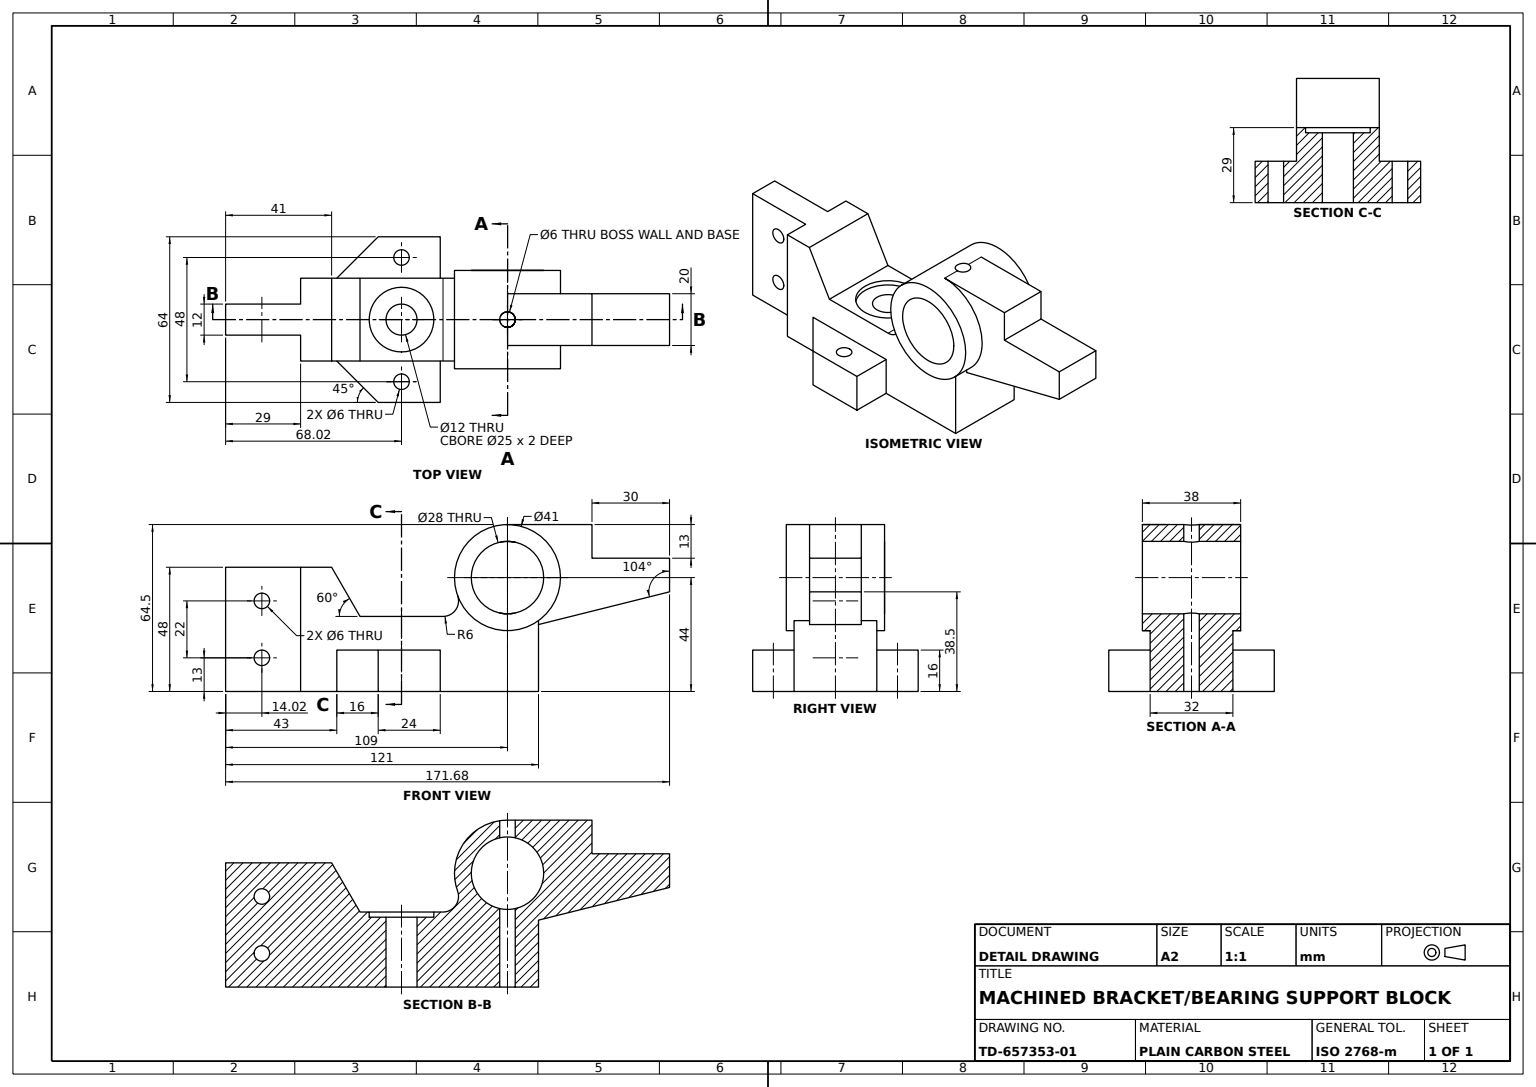
SolidWorks part; units mm, degrees
material "Plain Carbon Steel"
ref_plane "Front Plane" through (0, 0, 0) normal (0, 0, 1) x (1, 0, 0)
ref_plane "Top Plane" through (0, 0, 0) normal (0, 1, 0) x (1, 0, 0)
ref_plane "Right Plane" through (0, 0, 0) normal (1, 0, 0) x (0, 0, -1)
sketch "Base Block Sketch" plane through (0, 0, 0) normal (0, 0, 1) x (1, 0, 0)
  line L1 (-60.5, 24) -> (60.5, 24)
  line L2 (-60.5, 24) -> (-60.5, -24)
  line L3 (-60.5, -24) -> (60.5, -24)
  line L4 (60.5, 24) -> (60.5, -24)
  point P4 (0, -24)
  point P6 (-60.5, 0)
  dimension "D1" = 121
  dimension "D2" = 48
extrude "Base Block 121x48" add sketch "Base Block Sketch" along normal mid plane 32
sketch "Base Step Sketch" plane through (60.5, 0, 0) normal (1, 0, 0) x (0, 0, -1)
  line L0 (-16, -24) -> (16, -24) construction
  line L1 (-16, 24) -> (-6, 24)
  line L2 (-16, 24) -> (-16, -24)
  line L3 (-16, -24) -> (-6, -24)
  line L4 (-6, 24) -> (-6, -24)
  line L5 (0, 0) -> (0, 24) construction
  line L6 (16, 24) -> (6, 24)
  line L7 (16, 24) -> (16, -24)
  line L8 (16, -24) -> (6, -24)
  line L9 (6, 24) -> (6, -24)
  line L10 (-16, 24) -> (16, 24) construction
  dimension "D1" = 12
extrude "Base Step Cut" cut sketch "Base Step Sketch" against normal blind 29
sketch "Angled Relief Sketch" plane through (0, 0, 16) normal (0, 0, 1) x (1, 0, 0)
  line L0 (-60.5, 24) -> (-60.5, -24) construction
  line L1 (31.5, 24) -> (-60.5, 24) construction
  line L2 (19.5, 24) -> (8.5303, 5)
  line L3 (8.5303, 5) -> (-40, 5)
  line L4 (-40, 5) -> (-40, 24)
  line L5 (-60.5, -24) -> (31.5, -24) construction
  line L6 (31.5, 24) -> (31.5, -24) construction
  line L7 (-40, 24) -> (19.5, 24)
  dimension "D1" = 29
  dimension "D2" = 30
  dimension "D3" = 12
  dimension "D4" = 20.5
extrude "Angled Relief Cut 30deg" cut sketch "Angled Relief Sketch" against normal through all both and the other way through all
sketch "Pivot Boss Sketch" plane through (0, 0, 0) normal (0, 0, 1) x (1, 0, 0)
  line L0 (-60.5, -24) -> (31.5, -24) construction
  line L2 (-60.5, 24) -> (-60.5, -24) construction
  circle A0 centre (-48.5, 20) radius 20.5
  dimension "D3" = 41
  dimension "D1" = 44
  dimension "D2" = 12
extrude "Pivot Boss Ø44" add sketch "Pivot Boss Sketch" along normal mid plane 38
fillet "Pivot Boss Fillet R6" radius 6 1 edges at (-34.5268, 5, 0)
sketch "Clamp Tab Sketch" plane through (0, 0, 0) normal (0, 0, 1) x (1, 0, 0)
  line L0 (-48.5, 40.5) -> (-81.1788, 40.5)
  line L1 (-81.1788, 40.5) -> (-81.1788, 27.5)
  line L2 (-81.1788, 27.5) -> (-111.1788, 27.5)
  line L3 (-111.1788, 27.5) -> (-111.1788, 14.5)
  line L4 (-111.1788, 14.5) -> (-53.4594, 0.1089)
  circle A0 centre (-48.5, 20) radius 20.5 construction
  arc A1 (-48.5, 40.5) -> (-53.4594, 0.1089) centre (-48.5, 20) ccw
  dimension "D1" = 13
  dimension "D2" = 13
  dimension "D3" = 104
  dimension "D4" = 30
extrude "Clamp Tab" add sketch "Clamp Tab Sketch" along normal mid plane 20
sketch "Tab Pin Hole Sketch" plane through (0, 0, 0) normal (0, 1, 0) x (1, 0, 0)
  line L0 (-48.5, -10) -> (-48.5, 10) construction
  circle A0 centre (-48.5, 0) radius 3
  dimension "D1" = 6
extrude "Tab Pin Hole Ø6" cut sketch "Tab Pin Hole Sketch" against normal through all both and the other way through all
sketch "Pivot Bore Sketch" plane through (0, 0, 19) normal (0, 0, 1) x (1, 0, 0)
  circle A0 centre (-48.5, 20) radius 14
  dimension "D1" = 28
extrude "Pivot Bore Ø28" cut sketch "Pivot Bore Sketch" against normal through all both and the other way through all
hole_wizard "Counterbored Hole Ø12" positions "Sketch10" profile "Sketch11" legacy end condition up to next
sketch "Sketch10" plane through (0, 5, 0) normal (0, 1, 0) x (1, 0, 0)
  line L0 (-7.5224, 0) -> (-7.5224, -16) construction
  line L1 (-23.5751, -16) -> (8.5303, -16) construction
  point P0 (-7.5224, 0)
sketch "Sketch11" plane through (-7.5224, 5, 0) normal (1, 0, 0) x (0, 0, 1)
  line L0 (0, 0) -> (0, 29)
  line L1 (0, 29) -> (6, 29)
  line L2 (6, 29) -> (6, 2)
  line L3 (6, 2) -> (12.5, 2)
  line L4 (12.5, 2) -> (12.5, 0)
  line L5 (12.5, 0) -> (0, 0)
  line L6 (0, 110) -> (0, -10) construction
  dimension "Diameter" = 12
  dimension "Depth" = 29
  dimension "C-Bore Diameter" = 25
  dimension "C-Bore Depth" = 2
sketch "Mounting Flange Sketch" plane through (0, -24, 0) normal (0, -1, 0) x (1, 0, 0)
  line L0 (-22.5, -16) -> (-22.5, -32)
  line L1 (-60.5, -16) -> (31.5, -16) construction
  line L2 (-22.5, -32) -> (1.5, -32)
  line L3 (1.5, -32) -> (17.5, -16)
  line L4 (17.5, -16) -> (-22.5, -16)
  line L5 (-60.5, 16) -> (-60.5, -16) construction
  line L6 (0, 0) -> (-32.0998, 0) construction
  line L7 (17.5, 16) -> (-22.5, 16)
  line L8 (1.5, 32) -> (17.5, 16)
  line L9 (-22.5, 32) -> (1.5, 32)
  line L10 (-22.5, 16) -> (-22.5, 32)
  line L11 (-7.5224, -24) -> (-7.5224, -6) construction
  circle A0 centre (-7.5224, -24) radius 3
  circle A1 centre (-7.5224, 24) radius 3
  circle A2 centre (-7.5224, 0) radius 6 construction
  circle A3 centre (-7.5224, 0) radius 6 construction
  dimension "D5" = 6
  dimension "D1" = 38
  dimension "D2" = 24
  dimension "D3" = 16
  dimension "D4" = 16
  dimension "D6" = 48
extrude "Mounting Flange" add sketch "Mounting Flange Sketch" against normal blind 16
sketch "End Slot Sketch" plane through (0, 0, 6) normal (0, 0, 1) x (1, 0, 0)
  line L0 (0, 0) -> (60.5, 0) construction
  line L1 (60.5, -24) -> (60.5, 24) construction
  circle A0 centre (46.48, 11) radius 3
  circle A1 centre (46.48, -11) radius 3
  dimension "D2" = 6
  dimension "D1" = 22
  dimension "D3" = 46.48
extrude "End Slot Cut" cut sketch "End Slot Sketch" against normal through all both and the other way through all
